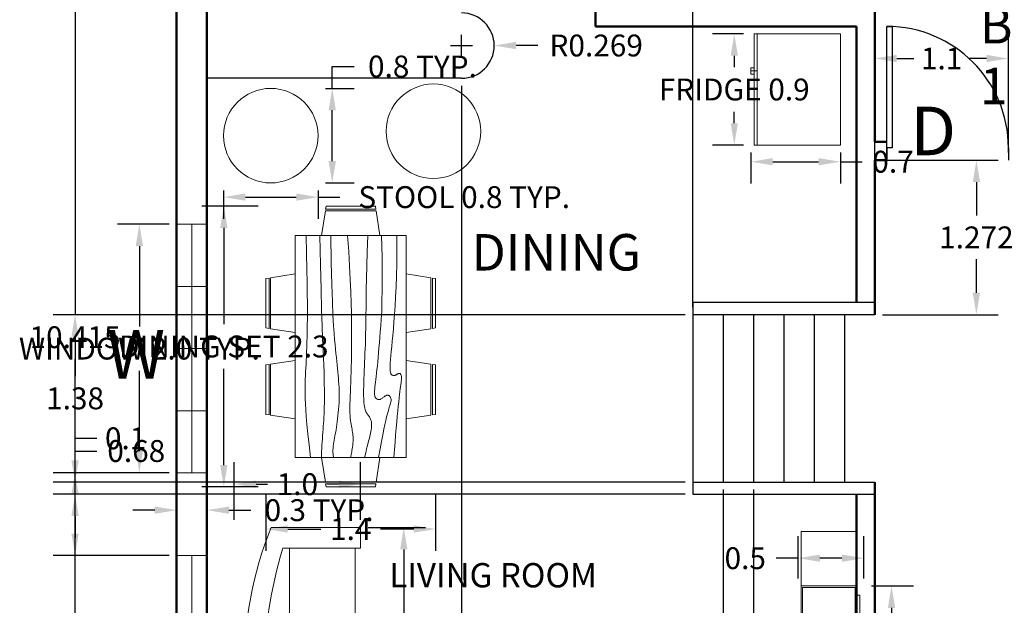
# Model space of a CAD drawing. Units: metres. Extents: x 3.9 to 21.3, y 24.8 to 56.5.
# Tile 4 of 6: x 4.9 to 13, y 31.2 to 36.1. Entities that reach past the tile are written whole.
import ezdxf

# ---------------------------------------------------------------- set-up
doc = ezdxf.new("R2010")
doc.units = ezdxf.units.M
doc.header["$MEASUREMENT"] = 0
for name, color, linetype, lineweight in [('A-AREA-IDEN', 3, 'Continuous', 25), ('A-EQPM', 6, 'Continuous', 18), ('A-FLOR-CASE', 8, 'Continuous', 25), ('A-FLOR-STRS', 7, 'Continuous', 25), ('DIMENSIONS', 2, 'Continuous', 18), ('DOOR', 5, 'Continuous', 25), ('FURNITURE', 6, 'Continuous', 18), ('TEXT', 3, 'Continuous', 18), ('WALL', 1, 'Continuous', 50), ('WINDOW', 4, 'Continuous', 18)]:
    doc.layers.add(name, color=color, linetype=linetype, lineweight=lineweight)
doc.styles.get("Standard").update_dxf_attribs({"font": 'arial.ttf'})
doc.dimstyles.get("Standard").update_dxf_attribs({"dimtxt": 0.18, "dimasz": 0.18, "dimexe": 0.18, "dimexo": 0.0625, "dimgap": 0.09, "dimtad": 0, "dimtih": 1, "dimtoh": 1, "dimdec": 1, "dimzin": 0, "dimdsep": 46, "dimtxsty": 'Standard', "dimcen": 0.09, "dimadec": 0, "dimazin": 0, "dimtfac": 1, "dimtdec": 1, "dimtofl": 0, "dimtmove": 0, "dimatfit": 3, "dimfxl": 1, "dimtolj": 1, "dimtzin": 0, "dimarcsym": 0})

# ---------------------------------------------------------------- blocks, each defined once
blk = doc.blocks.new('*U2')
for p, q in [((0, 0), (0, -100)), ((1000, 0), (1000, -100))]:
    blk.add_line(p, q)
blk.add_lwpolyline([(0, 0), (0, 1000), (43.75, 1000), (43.75, 0)], close=True)
blk.add_arc((0, 0), 1000, 0, 90)
blk = doc.blocks.new('Refrigerator-2 door - 36 in top')
for p, q in [((0, -26.999999), (36, -26.999999)), ((11, -27.999999), (11, -28.999999)), ((12, -26.999999), (12, -28.999999)), ((13, -28.999999), (13, -27.999999)), ((11, -28.999999), (13, -28.999999))]:
    blk.add_line(p, q)
blk.add_lwpolyline([(0, -27.999999), (0, 0), (36, 0), (36, -27.999999)], close=True)
blk = doc.blocks.new('Dining Set - 36 x 72 in.')
for p, q in [((-22.2343, 26.00059), (-23.4847, 17.99762)), ((-22.2304, 26), (-5.7608, 26)), ((-22, 27.5), (-22.1562, 26.50042)), ((-5.8416, 26.5), (-22.1534, 26.5)), ((-22, 27.5), (-6, 27.5)), ((-5.8437, 26.49966), (-6, 27.5)), ((-4.5152, 17.99762), (-5.7655, 25.99926)), ((5.7657, 26.00059), (4.5153, 17.99762)), ((5.7696, 26), (22.2392, 26)), ((6, 27.5), (5.8438, 26.50042)), ((22.1584, 26.5), (5.8466, 26.5)), ((6, 27.5), (22, 27.5)), ((22.1563, 26.49966), (22, 27.5)), ((23.4848, 17.99762), (22.2345, 25.99926)), ((36, 18), (-36, 18)), ((-36, 18), (-36, -18)), ((36, -18), (36, 18)), ((-45.5, 8), (-44.5004, 8.15617)), ((-45.5, 8), (-45.5, -8)), ((-44.5, -8.15843), (-44.5, 8.15338)), ((-44.0006, 8.23428), (-35.9976, 9.48474)), ((-44, 8.23041), (-44, -8.23915)), ((44.0006, 8.23428), (35.9976, 9.48474)), ((44, 8.23041), (44, -8.23915)), ((44.5, -8.15843), (44.5, 8.15338)), ((45.5, 8), (44.5005, 8.15617)), ((45.5, 8), (45.5, -8)), ((-44.4997, -8.15631), (-45.5, -8)), ((-35.9976, -9.48476), (-43.9993, -8.2345)), ((35.9976, -9.48476), (43.9993, -8.2345)), ((44.4997, -8.15631), (45.5, -8)), ((-36, -18), (36, -18)), ((-22.2343, -26.0006), (-23.4847, -17.99762)), ((-4.5152, -17.99762), (-5.7655, -25.99928)), ((5.7657, -26.0006), (4.5153, -17.99762)), ((23.4848, -17.99762), (22.2345, -25.99928)), ((-22.2304, -26), (-5.7608, -26)), ((-22, -27.5), (-22.1562, -26.50044)), ((-5.8416, -26.5), (-22.1534, -26.5)), ((-22, -27.5), (-6, -27.5)), ((-5.8437, -26.49967), (-6, -27.5)), ((5.7696, -26), (22.2392, -26)), ((6, -27.5), (5.8438, -26.50044)), ((22.1584, -26.5), (5.8466, -26.5)), ((6, -27.5), (22, -27.5)), ((22.1563, -26.49967), (22, -27.5))]:
    blk.add_line(p, q)
for points in [[(-36, 15), (-31.1772, 14.97754), (-26.8079, 14.91406), (-22.8538, 14.81543), (-19.276, 14.6875), (-16.0362, 14.53613), (-13.0957, 14.36718), (-10.4159, 14.18652), (-7.9583, 14), (-5.6904, 13.81315), (-3.6035, 13.63021), (-1.6954, 13.45508), (0.0365, 13.29166), (1.5945, 13.14388), (2.9811, 13.01562), (4.1988, 12.9108), (5.25, 12.83333), (6.1393, 12.78613), (6.8802, 12.76823), (7.4883, 12.77767), (7.9792, 12.8125), (8.3685, 12.87077), (8.6719, 12.95052), (8.9049, 13.0498), (9.0833, 13.16666), (9.2205, 13.29899), (9.3216, 13.44401), (9.3895, 13.59879), (9.4271, 13.76041), (9.4373, 13.92594), (9.4232, 14.09245), (9.3875, 14.257), (9.3333, 14.41666), (9.2638, 14.56917), (9.1836, 14.71484), (9.0975, 14.85465), (9.0104, 14.98958), (8.9272, 15.1206), (8.8529, 15.2487), (8.7922, 15.37483), (8.75, 15.5), (8.7305, 15.62467), (8.7344, 15.74739), (8.7617, 15.86621), (8.8125, 15.97916), (8.8867, 16.08431), (8.9844, 16.17968), (9.1055, 16.26334), (9.25, 16.33333), (9.4189, 16.38802), (9.6172, 16.42708), (9.8506, 16.45052), (10.125, 16.45833), (10.4463, 16.45052), (10.8203, 16.42708), (11.2529, 16.38802), (11.75, 16.33333), (12.3184, 16.26318), (12.9694, 16.17838), (13.7151, 16.07991), (14.5677, 15.96875), (15.5395, 15.84586), (16.6426, 15.71224), (17.8893, 15.56884), (19.2917, 15.41666), (20.859, 15.25667), (22.5879, 15.08984), (24.4721, 14.91715), (26.5052, 14.73958), (28.6809, 14.5581), (30.9929, 14.3737), (33.4347, 14.18733), (36, 14)], [(-36, 10), (-28.9766, 10.14274), (-23.1725, 10.20442), (-18.4241, 10.19775), (-14.5677, 10.13541), (-11.4399, 10.03011), (-8.877, 9.89453), (-6.7154, 9.74137), (-4.7917, 9.58333), (-2.9698, 9.43082), (-1.2246, 9.28515), (0.4415, 9.14534), (2.026, 9.01041), (3.5266, 8.87939), (4.9408, 8.7513), (6.266, 8.62516), (7.5, 8.5), (8.6411, 8.37549), (9.6914, 8.2539), (10.6538, 8.13818), (11.5312, 8.03125), (12.3267, 7.93603), (13.043, 7.85547), (13.6831, 7.79248), (14.25, 7.75), (14.7471, 7.7303), (15.1797, 7.73307), (15.5537, 7.75732), (15.875, 7.80208), (16.1494, 7.86637), (16.3828, 7.94922), (16.5811, 8.04964), (16.75, 8.16666), (16.8944, 8.29915), (17.0143, 8.44531), (17.1089, 8.60319), (17.1771, 8.77083), (17.218, 8.94629), (17.2305, 9.1276), (17.2137, 9.31282), (17.1667, 9.5), (17.0895, 9.6875), (16.987, 9.875), (16.8649, 10.0625), (16.7292, 10.25), (16.5856, 10.4375), (16.4401, 10.625), (16.2985, 10.8125), (16.1667, 11), (16.05, 11.18733), (15.9518, 11.3737), (15.8752, 11.5581), (15.8229, 11.73958), (15.798, 11.91715), (15.8034, 12.08984), (15.842, 12.25667), (15.9167, 12.41666), (16.0295, 12.56836), (16.1784, 12.70833), (16.3605, 12.83268), (16.5729, 12.9375), (16.8127, 13.01888), (17.0768, 13.07291), (17.3625, 13.0957), (17.6667, 13.08333), (17.9894, 13.03312), (18.3418, 12.94726), (18.7382, 12.82918), (19.1927, 12.68229), (19.7195, 12.51001), (20.3327, 12.31575), (21.0465, 12.10294), (21.875, 11.875), (22.8357, 11.63354), (23.959, 11.37304), (25.2786, 11.08618), (26.8282, 10.76562), (28.6414, 10.40405), (30.752, 9.99414), (33.1936, 9.52856), (36, 9)], [(-36, 5.5), (-30.7157, 5.3348), (-26.069, 5.20963), (-21.9946, 5.11767), (-18.4271, 5.05208), (-15.3009, 5.00602), (-12.5508, 4.97265), (-10.1112, 4.94515), (-7.9167, 4.91666), (-5.909, 4.88167), (-4.0586, 4.83984), (-2.3429, 4.79215), (-0.7396, 4.73958), (0.7739, 4.6831), (2.22, 4.6237), (3.6213, 4.56233), (5, 4.5), (6.373, 4.43782), (7.7344, 4.3776), (9.0723, 4.32129), (10.375, 4.27083), (11.6309, 4.22819), (12.8281, 4.19531), (13.9551, 4.17415), (15, 4.16666), (15.954, 4.17448), (16.819, 4.19791), (17.6001, 4.23698), (18.3021, 4.29166), (18.9299, 4.36198), (19.4883, 4.44791), (19.9823, 4.54948), (20.4167, 4.66666), (20.7969, 4.79899), (21.1302, 4.94401), (21.4245, 5.09879), (21.6875, 5.26041), (21.9271, 5.42594), (22.1511, 5.59245), (22.3672, 5.757), (22.5834, 5.91666), (22.8065, 6.06868), (23.0404, 6.21093), (23.2879, 6.34147), (23.5521, 6.45833), (23.8358, 6.55957), (24.142, 6.64323), (24.4735, 6.70735), (24.8334, 6.75), (25.2235, 6.76969), (25.642, 6.76692), (26.0858, 6.74267), (26.5521, 6.69791), (27.0379, 6.63362), (27.5404, 6.55078), (28.0565, 6.45036), (28.5834, 6.33333), (29.1242, 6.19987), (29.7071, 6.04687), (30.3661, 5.87044), (31.1354, 5.66666), (32.0493, 5.43164), (33.142, 5.16146), (34.4475, 4.85221), (36, 4.5)], [(-36, -1), (-30.7915, -0.6591), (-26.0195, -0.38216), (-21.6519, -0.16284), (-17.6563, 0.00521), (-14.0005, 0.12833), (-10.6523, 0.21289), (-7.5796, 0.26522), (-4.75, 0.29166), (-2.134, 0.29793), (0.2878, 0.28711), (2.5317, 0.26163), (4.6146, 0.22396), (6.5529, 0.17651), (8.3633, 0.12174), (10.0623, 0.06209), (11.6667, 0), (13.1899, -0.06201), (14.6341, -0.1211), (15.9982, -0.17432), (17.2813, -0.21875), (18.4823, -0.25147), (19.6003, -0.26953), (20.6343, -0.27002), (21.5834, -0.25), (22.4481, -0.20768), (23.2357, -0.14584), (23.9549, -0.06836), (24.6146, 0.02083), (25.2235, 0.11784), (25.7904, 0.21875), (26.3241, 0.31966), (26.8334, 0.41666), (27.3265, 0.50618), (27.8099, 0.58593), (28.2894, 0.65397), (28.7709, 0.70833), (29.2601, 0.74707), (29.763, 0.76823), (30.2855, 0.76985), (30.8334, 0.75), (31.4088, 0.70784), (31.9994, 0.64713), (32.589, 0.57275), (33.1615, 0.48958), (33.7008, 0.4025), (34.1908, 0.3164), (34.6153, 0.23616), (34.9584, 0.16666), (35.2099, 0.11165), (35.3848, 0.07031), (35.504, 0.04069), (35.5886, 0.02083), (35.6594, 0.00879), (35.7377, 0.0026), (35.8442, 0.00032), (36, 0)], [(-36, -6.5), (-27.1843, -6.31267), (-20.084, -6.1263), (-14.469, -5.9419), (-10.1094, -5.76042), (-6.7752, -5.58285), (-4.2363, -5.41016), (-2.2629, -5.24333), (-0.625, -5.08334), (0.8708, -4.93099), (2.2715, -4.78646), (3.5872, -4.64974), (4.8281, -4.52084), (6.0046, -4.39974), (7.127, -4.28646), (8.2053, -4.18099), (9.25, -4.08334), (10.2705, -3.99382), (11.2734, -3.91407), (12.2647, -3.84603), (13.25, -3.79167), (14.2354, -3.75293), (15.2266, -3.73177), (16.2295, -3.73015), (17.25, -3.75), (18.2912, -3.79248), (19.3451, -3.85547), (20.4009, -3.93604), (21.4479, -4.03125), (22.4754, -4.13819), (23.4727, -4.25391), (24.4289, -4.37549), (25.3334, -4.5), (26.1785, -4.62492), (26.9694, -4.74935), (27.7145, -4.87281), (28.4219, -4.99479), (29.1, -5.11483), (29.7572, -5.23242), (30.4016, -5.34709), (31.0417, -5.45834), (31.6837, -5.56437), (32.3262, -5.65821), (32.9658, -5.73153), (33.599, -5.77604), (34.2224, -5.78345), (34.8327, -5.74545), (35.4264, -5.65373), (36, -5.5)], [(-36, -10), (-26.4022, -9.81299), (-18.4675, -9.62891), (-11.9839, -9.45069), (-6.7396, -9.28125), (-2.5226, -9.12354), (0.8789, -8.98047), (3.6769, -8.85498), (6.0833, -8.75), (8.2767, -8.66765), (10.3021, -8.60677), (12.1712, -8.56543), (13.8958, -8.54167), (15.4876, -8.53353), (16.9583, -8.53907), (18.3197, -8.55632), (19.5834, -8.58334), (20.7616, -8.61841), (21.8685, -8.66081), (22.9188, -8.71004), (23.9271, -8.76563), (24.9081, -8.82707), (25.8763, -8.89388), (26.8465, -8.96558), (27.8334, -9.04167), (28.8474, -9.12118), (29.8828, -9.20117), (30.93, -9.27824), (31.9792, -9.34896), (33.0205, -9.40991), (34.0443, -9.45768), (35.0407, -9.48885), (36, -9.5)], [(-36, -14.5), (-30.0881, -14.33513), (-25.0332, -14.21224), (-20.7312, -14.12647), (-17.0781, -14.07292), (-13.97, -14.04671), (-11.3027, -14.04297), (-8.9724, -14.05681), (-6.875, -14.08334), (-4.9224, -14.11833), (-3.0905, -14.16016), (-1.3709, -14.20785), (0.2448, -14.26042), (1.7647, -14.3169), (3.1973, -14.3763), (4.5507, -14.43767), (5.8333, -14.5), (7.0554, -14.5621), (8.235, -14.62175), (9.3922, -14.67652), (10.5469, -14.72396), (11.7192, -14.76164), (12.929, -14.78711), (14.1965, -14.79794), (15.5417, -14.79167), (16.9933, -14.76424), (18.6152, -14.70508), (20.4804, -14.60197), (22.6615, -14.44271), (25.2312, -14.21509), (28.2624, -13.9069), (31.8277, -13.50594), (36, -13)]]:
    blk.add_lwpolyline(points)
blk = doc.blocks.new('Entertainment Center')
for p, q in [((-4, 0), (-5, -1)), ((4, 0), (-4, 0)), ((5, -1), (4, 0)), ((-17, -19), (-17, -1)), ((-17, -1), (43, -1)), ((-16.5, -18.5), (-16.5, -1.5)), ((-16.5, -1.5), (42.5, -1.5)), ((42.5, -1.5), (42.5, -18.5)), ((43, -1), (43, -19)), ((43, -19), (-17, -19)), ((42.5, -18.5), (-16.5, -18.5)), ((-12, -20), (-12, -19)), ((12, -19), (12, -20)), ((15, -20), (15, -19)), ((27, -19), (27, -20)), ((28, -20), (28, -19)), ((40, -19), (40, -20)), ((12, -20), (-12, -20)), ((27, -20), (15, -20)), ((40, -20), (28, -20))]:
    blk.add_line(p, q)
blk.add_arc((0, 40), 61, 259.6111, 280.3889)
blk = doc.blocks.new('Sofa - Roundback 7 ft.')
for p, q in [((-12.00002, -32.4421), (-12.00003, -6.5971)), ((11.99997, -32.4421), (11.99998, -6.5971)), ((-36.000027, -34), (-36.000027, -11.4696)), ((-35.999844, -13.3819), (35.9998, -13.3819)), ((35.99998, -34), (35.99998, -11.4696)), ((-36.000027, -32.4421), (35.99998, -32.4421))]:
    blk.add_line(p, q)
for points in [[(-36.000027, -34), (-42.000027, -34), (-42.000027, -8)], [(41.99998, -8), (41.99998, -34), (35.99998, -34)]]:
    blk.add_lwpolyline(points)
for centre, radius, start, end in [((0, -114.25), 114.25, 68.43141, 111.5686), ((-0.00001, -127.1968), 121.1968, 72.72033, 107.2797)]:
    blk.add_arc(centre, radius, start, end)
blk = doc.blocks.new('WIN-4-LIGHT-2046')
for p, q in [((0.5115, -0.125), (0, -0.125)), ((0.5115, -0.125), (1.0231, -0.125)), ((1.5346, -0.125), (1.0231, -0.125)), ((1.5346, -0.125), (2.0462, -0.125))]:
    blk.add_line(p, q)
for points in [[(0.5115, 0), (0, 0), (0, -0.25), (0.5115, -0.25)], [(0.5115, 0), (1.0231, 0), (1.0231, -0.25), (0.5115, -0.25)], [(1.5346, 0), (1.0231, 0), (1.0231, -0.25), (1.5346, -0.25)], [(1.5346, 0), (2.0462, 0), (2.0462, -0.25), (1.5346, -0.25)]]:
    blk.add_lwpolyline(points, close=True)
blk = doc.blocks.new('STOOL-ROUND-778')
blk.add_circle((0, 0), 0.3891)
blk = doc.blocks.new('*D37')
at = {"layer": 'Defpoints', "color": 0, "transparency": 16777216}
for p in [(6.1571, 34.3672), (5.8502, 32.321), (6.1571, 32.321)]:
    blk.add_point(p, dxfattribs=at)
at = {"layer": 'DIMENSIONS', "color": 0, "lineweight": -2, "transparency": 16777216}
for p, q in [((6.0946, 34.3672), (5.6702, 34.3672)), ((5.8502, 34.1872), (5.8502, 33.5272)), ((5.8502, 32.501), (5.8502, 33.161)), ((6.0946, 32.321), (5.6702, 32.321))]:
    blk.add_line(p, q, dxfattribs=at)
at = {"layer": 'DIMENSIONS', "color": 0, "transparency": 16777216}
for points in [[(5.8202, 34.1872), (5.8802, 34.1872), (5.8502, 34.3672)], [(5.8202, 32.501), (5.8802, 32.501), (5.8502, 32.321)]]:
    blk.add_solid(points, dxfattribs=at)
at = {"layer": 'DIMENSIONS', "color": 0, "transparency": 16777216, "insert": (5.8502, 33.3441), "char_height": 0.18, "attachment_point": 5}
blk.add_mtext('\\A1;WINDOW 2.0 TYP.', dxfattribs=at)
blk = doc.blocks.new('*D38')
at = {"layer": 'Defpoints', "color": 0, "transparency": 16777216}
for p in [(6.1571, 32.321), (6.4071, 32.321), (6.4071, 32.0141)]:
    blk.add_point(p, dxfattribs=at)
at = {"layer": 'DIMENSIONS', "color": 0, "lineweight": -2, "transparency": 16777216}
for p, q in [((6.1571, 32.2585), (6.1571, 31.8341)), ((6.4071, 32.2585), (6.4071, 31.8341)), ((5.9771, 32.0141), (5.7971, 32.0141)), ((6.5871, 32.0141), (6.7671, 32.0141))]:
    blk.add_line(p, q, dxfattribs=at)
at = {"layer": 'DIMENSIONS', "color": 0, "transparency": 16777216}
for points in [[(5.9771, 32.0441), (5.9771, 31.9841), (6.1571, 32.0141)], [(6.5871, 32.0441), (6.5871, 31.9841), (6.4071, 32.0141)]]:
    blk.add_solid(points, dxfattribs=at)
at = {"layer": 'DIMENSIONS', "color": 0, "transparency": 16777216, "insert": (7.3301, 32.0141), "char_height": 0.18, "attachment_point": 5}
blk.add_mtext('\\A1;0.3 TYP.', dxfattribs=at)
blk = doc.blocks.new('*D49')
at = {"layer": 'Defpoints', "color": 0, "transparency": 16777216}
for p in [(6.5435, 34.7074), (7.3217, 34.7074), (7.3217, 34.5907)]:
    blk.add_point(p, dxfattribs=at)
at = {"layer": 'DIMENSIONS', "color": 0, "lineweight": -2, "transparency": 16777216}
for p, q in [((6.5435, 34.6449), (6.5435, 34.4107)), ((7.3217, 34.6449), (7.3217, 34.4107)), ((6.7235, 34.5907), (7.1417, 34.5907)), ((7.3217, 34.5907), (7.5017, 34.5907))]:
    blk.add_line(p, q, dxfattribs=at)
at = {"layer": 'DIMENSIONS', "color": 0, "transparency": 16777216}
for points in [[(6.7235, 34.6207), (6.7235, 34.5607), (6.5435, 34.5907)], [(7.1417, 34.6207), (7.1417, 34.5607), (7.3217, 34.5907)]]:
    blk.add_solid(points, dxfattribs=at)
at = {"layer": 'DIMENSIONS', "color": 0, "transparency": 16777216, "insert": (8.5254, 34.5907), "char_height": 0.18, "attachment_point": 5}
blk.add_mtext('\\A1;STOOL 0.8 TYP.', dxfattribs=at)
blk = doc.blocks.new('*D50')
at = {"layer": 'Defpoints', "color": 0, "transparency": 16777216}
for p in [(7.3217, 35.4856), (7.4385, 35.4856), (7.3217, 34.7074)]:
    blk.add_point(p, dxfattribs=at)
at = {"layer": 'DIMENSIONS', "color": 0, "lineweight": -2, "transparency": 16777216}
for p, q in [((7.4385, 35.4856), (7.4385, 35.6656)), ((7.4385, 35.6656), (7.6185, 35.6656)), ((7.3842, 35.4856), (7.6185, 35.4856)), ((7.4385, 34.8874), (7.4385, 35.3056)), ((7.3842, 34.7074), (7.6185, 34.7074))]:
    blk.add_line(p, q, dxfattribs=at)
at = {"layer": 'DIMENSIONS', "color": 0, "transparency": 16777216}
for points in [[(7.4085, 35.3056), (7.4685, 35.3056), (7.4385, 35.4856)], [(7.4085, 34.8874), (7.4685, 34.8874), (7.4385, 34.7074)]]:
    blk.add_solid(points, dxfattribs=at)
at = {"layer": 'DIMENSIONS', "color": 0, "transparency": 16777216, "insert": (8.1815, 35.6656), "char_height": 0.18, "attachment_point": 5}
blk.add_mtext('\\A1;0.8 TYP.', dxfattribs=at)
blk = doc.blocks.new('*D51')
at = {"layer": 'Defpoints', "color": 0, "transparency": 16777216}
for p in [(10.8867, 35.9335), (10.7495, 35.0191), (10.8867, 35.0191)]:
    blk.add_point(p, dxfattribs=at)
at = {"layer": 'DIMENSIONS', "color": 0, "lineweight": -2, "transparency": 16777216}
for p, q in [((10.8242, 35.9335), (10.5695, 35.9335)), ((10.7495, 35.7535), (10.7495, 35.6594)), ((10.7495, 35.1991), (10.7495, 35.2933)), ((10.8242, 35.0191), (10.5695, 35.0191))]:
    blk.add_line(p, q, dxfattribs=at)
at = {"layer": 'DIMENSIONS', "color": 0, "transparency": 16777216}
for points in [[(10.7195, 35.7535), (10.7795, 35.7535), (10.7495, 35.9335)], [(10.7195, 35.1991), (10.7795, 35.1991), (10.7495, 35.0191)]]:
    blk.add_solid(points, dxfattribs=at)
at = {"layer": 'DIMENSIONS', "color": 0, "transparency": 16777216, "insert": (10.7495, 35.4763), "char_height": 0.18, "attachment_point": 5}
blk.add_mtext('\\A1;FRIDGE 0.9', dxfattribs=at)
blk = doc.blocks.new('*D52')
at = {"layer": 'Defpoints', "color": 0, "transparency": 16777216}
for p in [(10.8867, 35.0191), (11.6233, 35.0191), (11.6233, 34.882)]:
    blk.add_point(p, dxfattribs=at)
at = {"layer": 'DIMENSIONS', "color": 0, "lineweight": -2, "transparency": 16777216}
for p, q in [((10.8867, 34.9566), (10.8867, 34.702)), ((11.6233, 34.9566), (11.6233, 34.702)), ((11.0667, 34.882), (11.4433, 34.882)), ((11.6233, 34.882), (11.8033, 34.882))]:
    blk.add_line(p, q, dxfattribs=at)
at = {"layer": 'DIMENSIONS', "color": 0, "transparency": 16777216}
for points in [[(11.0667, 34.912), (11.0667, 34.852), (10.8867, 34.882)], [(11.4433, 34.912), (11.4433, 34.852), (11.6233, 34.882)]]:
    blk.add_solid(points, dxfattribs=at)
at = {"layer": 'DIMENSIONS', "color": 0, "transparency": 16777216, "insert": (12.0571, 34.882), "char_height": 0.18, "attachment_point": 5}
blk.add_mtext('\\A1;0.7', dxfattribs=at)
blk = doc.blocks.new('*D57')
at = {"layer": 'Defpoints', "color": 0, "transparency": 16777216}
for p in [(6.8924, 34.5172), (6.5457, 32.2058), (6.8924, 32.2058)]:
    blk.add_point(p, dxfattribs=at)
at = {"layer": 'DIMENSIONS', "color": 0, "lineweight": -2, "transparency": 16777216}
for p, q in [((6.8299, 34.5172), (6.3657, 34.5172)), ((6.5457, 34.3372), (6.5457, 33.5447)), ((6.5457, 32.3858), (6.5457, 33.1784)), ((6.8299, 32.2058), (6.3657, 32.2058))]:
    blk.add_line(p, q, dxfattribs=at)
at = {"layer": 'DIMENSIONS', "color": 0, "transparency": 16777216}
for points in [[(6.5157, 34.3372), (6.5757, 34.3372), (6.5457, 34.5172)], [(6.5157, 32.3858), (6.5757, 32.3858), (6.5457, 32.2058)]]:
    blk.add_solid(points, dxfattribs=at)
at = {"layer": 'DIMENSIONS', "color": 0, "transparency": 16777216, "insert": (6.5457, 33.3615), "char_height": 0.18, "attachment_point": 5}
blk.add_mtext('\\A1;DINING SET 2.3', dxfattribs=at)
blk = doc.blocks.new('*D58')
at = {"layer": 'Defpoints', "color": 0, "transparency": 16777216}
for p in [(6.8924, 32.2058), (8.2894, 32.2058), (8.2894, 31.8591)]:
    blk.add_point(p, dxfattribs=at)
at = {"layer": 'DIMENSIONS', "color": 0, "lineweight": -2, "transparency": 16777216}
for p, q in [((6.8924, 32.1433), (6.8924, 31.6791)), ((8.2894, 32.1433), (8.2894, 31.6791)), ((7.0724, 31.8591), (7.3459, 31.8591)), ((8.1094, 31.8591), (7.8359, 31.8591))]:
    blk.add_line(p, q, dxfattribs=at)
at = {"layer": 'DIMENSIONS', "color": 0, "transparency": 16777216}
for points in [[(7.0724, 31.8891), (7.0724, 31.8291), (6.8924, 31.8591)], [(8.1094, 31.8891), (8.1094, 31.8291), (8.2894, 31.8591)]]:
    blk.add_solid(points, dxfattribs=at)
at = {"layer": 'DIMENSIONS', "color": 0, "transparency": 16777216, "insert": (7.5909, 31.8591), "char_height": 0.18, "attachment_point": 5}
blk.add_mtext('\\A1;1.4', dxfattribs=at)
blk = doc.blocks.new('*D59')
at = {"layer": 'Defpoints', "color": 0, "transparency": 16777216}
for p in [(11.8164, 31.3903), (12.045, 31.3903), (11.8164, 29.8663)]:
    blk.add_point(p, dxfattribs=at)
at = {"layer": 'DIMENSIONS', "color": 0, "lineweight": -2, "transparency": 16777216}
for p, q in [((11.8789, 31.3903), (12.225, 31.3903)), ((12.045, 31.2103), (12.045, 30.8102)), ((12.045, 30.0463), (12.045, 30.4464)), ((11.8789, 29.8663), (12.225, 29.8663))]:
    blk.add_line(p, q, dxfattribs=at)
at = {"layer": 'DIMENSIONS', "color": 0, "transparency": 16777216}
for points in [[(12.015, 31.2103), (12.075, 31.2103), (12.045, 31.3903)], [(12.015, 30.0463), (12.075, 30.0463), (12.045, 29.8663)]]:
    blk.add_solid(points, dxfattribs=at)
at = {"layer": 'DIMENSIONS', "color": 0, "transparency": 16777216, "insert": (12.045, 30.6283), "char_height": 0.18, "attachment_point": 5}
blk.add_mtext('\\A1;MEDIA UNIT 1.5', dxfattribs=at)
blk = doc.blocks.new('*D60')
at = {"layer": 'Defpoints', "color": 0, "transparency": 16777216}
for p in [(11.2746, 31.6189), (11.2746, 31.3903), (11.8164, 31.3903)]:
    blk.add_point(p, dxfattribs=at)
at = {"layer": 'DIMENSIONS', "color": 0, "lineweight": -2, "transparency": 16777216}
for p, q in [((11.2746, 31.4528), (11.2746, 31.7989)), ((11.8164, 31.4528), (11.8164, 31.7989)), ((11.2746, 31.6189), (11.0946, 31.6189)), ((11.6364, 31.6189), (11.4546, 31.6189))]:
    blk.add_line(p, q, dxfattribs=at)
at = {"layer": 'DIMENSIONS', "color": 0, "transparency": 16777216}
for points in [[(11.4546, 31.6489), (11.4546, 31.5889), (11.2746, 31.6189)], [(11.6364, 31.6489), (11.6364, 31.5889), (11.8164, 31.6189)]]:
    blk.add_solid(points, dxfattribs=at)
at = {"layer": 'DIMENSIONS', "color": 0, "transparency": 16777216, "insert": (10.84, 31.6189), "char_height": 0.18, "attachment_point": 5}
blk.add_mtext('\\A1;0.5', dxfattribs=at)
blk = doc.blocks.new('*D61')
at = {"layer": 'Defpoints', "color": 0, "transparency": 16777216}
for p in [(7.6708, 31.8712), (8.0277, 31.8712), (7.6708, 29.4918)]:
    blk.add_point(p, dxfattribs=at)
at = {"layer": 'DIMENSIONS', "color": 0, "lineweight": -2, "transparency": 16777216}
for p, q in [((7.7333, 31.8712), (8.2077, 31.8712)), ((8.0277, 31.6912), (8.0277, 30.8646)), ((8.0277, 29.6718), (8.0277, 30.4984)), ((7.7333, 29.4918), (8.2077, 29.4918))]:
    blk.add_line(p, q, dxfattribs=at)
at = {"layer": 'DIMENSIONS', "color": 0, "transparency": 16777216}
for points in [[(7.9977, 31.6912), (8.0577, 31.6912), (8.0277, 31.8712)], [(7.9977, 29.6718), (8.0577, 29.6718), (8.0277, 29.4918)]]:
    blk.add_solid(points, dxfattribs=at)
at = {"layer": 'DIMENSIONS', "color": 0, "transparency": 16777216, "insert": (8.0277, 30.6815), "char_height": 0.18, "attachment_point": 5}
blk.add_mtext('\\A1;SOFA 2.4', dxfattribs=at)
blk = doc.blocks.new('*D62')
at = {"layer": 'Defpoints', "color": 0, "transparency": 16777216}
for p in [(6.6321, 32.2281), (6.6321, 31.8712), (7.6708, 31.8712)]:
    blk.add_point(p, dxfattribs=at)
at = {"layer": 'DIMENSIONS', "color": 0, "lineweight": -2, "transparency": 16777216}
for p, q in [((6.6321, 31.9337), (6.6321, 32.4081)), ((7.6708, 31.9337), (7.6708, 32.4081)), ((6.8121, 32.2281), (6.9064, 32.2281)), ((7.4908, 32.2281), (7.3965, 32.2281))]:
    blk.add_line(p, q, dxfattribs=at)
at = {"layer": 'DIMENSIONS', "color": 0, "transparency": 16777216}
for points in [[(6.8121, 32.2581), (6.8121, 32.1981), (6.6321, 32.2281)], [(7.4908, 32.2581), (7.4908, 32.1981), (7.6708, 32.2281)]]:
    blk.add_solid(points, dxfattribs=at)
at = {"layer": 'DIMENSIONS', "color": 0, "transparency": 16777216, "insert": (7.1514, 32.2281), "char_height": 0.18, "attachment_point": 5}
blk.add_mtext('\\A1;1.0', dxfattribs=at)
blk = doc.blocks.new('*D65')
at = {"layer": 'Defpoints', "color": 0, "transparency": 16777216}
for p in [(9.0686, 30.8635), (9.1864, 30.8635), (9.0686, 30.0783)]:
    blk.add_point(p, dxfattribs=at)
at = {"layer": 'DIMENSIONS', "color": 0, "lineweight": -2, "transparency": 16777216}
for p, q in [((9.1864, 30.8635), (9.1864, 31.0435)), ((9.1864, 31.0435), (9.3664, 31.0435)), ((9.1311, 30.8635), (9.3664, 30.8635)), ((9.1864, 30.2583), (9.1864, 30.6835)), ((9.1311, 30.0783), (9.3664, 30.0783))]:
    blk.add_line(p, q, dxfattribs=at)
at = {"layer": 'DIMENSIONS', "color": 0, "transparency": 16777216}
for points in [[(9.1564, 30.6835), (9.2164, 30.6835), (9.1864, 30.8635)], [(9.1564, 30.2583), (9.2164, 30.2583), (9.1864, 30.0783)]]:
    blk.add_solid(points, dxfattribs=at)
at = {"layer": 'DIMENSIONS', "color": 0, "transparency": 16777216, "insert": (10.5975, 31.0435), "char_height": 0.18, "attachment_point": 5}
blk.add_mtext('\\A1;COFFEE TABLE 0.8', dxfattribs=at)
blk = doc.blocks.new('*D75')
at = {"layer": 'Defpoints', "color": 0, "transparency": 16777216}
for p in [(13.0071, 35.7316), (11.9071, 34.8951), (13.0071, 34.8951)]:
    blk.add_point(p, dxfattribs=at)
at = {"layer": 'DIMENSIONS', "color": 0, "lineweight": -2, "transparency": 16777216}
for p, q in [((11.9071, 34.9576), (11.9071, 35.9116)), ((13.0071, 34.9576), (13.0071, 35.9116)), ((12.0871, 35.7316), (12.2291, 35.7316)), ((12.8271, 35.7316), (12.6851, 35.7316))]:
    blk.add_line(p, q, dxfattribs=at)
at = {"layer": 'DIMENSIONS', "color": 0, "transparency": 16777216}
for points in [[(12.0871, 35.7616), (12.0871, 35.7016), (11.9071, 35.7316)], [(12.8271, 35.7616), (12.8271, 35.7016), (13.0071, 35.7316)]]:
    blk.add_solid(points, dxfattribs=at)
at = {"layer": 'DIMENSIONS', "color": 0, "transparency": 16777216, "insert": (12.4571, 35.7316), "char_height": 0.18, "attachment_point": 5}
blk.add_mtext('\\A1;1.1', dxfattribs=at)
blk = doc.blocks.new('*D76')
at = {"layer": 'Defpoints', "color": 0, "transparency": 16777216}
for p in [(6.4071, 38.6451), (5.3206, 28.2303), (6.4071, 28.2303)]:
    blk.add_point(p, dxfattribs=at)
at = {"layer": 'DIMENSIONS', "color": 0, "lineweight": -2, "transparency": 16777216}
for p, q in [((6.3446, 38.6451), (5.1406, 38.6451)), ((5.3206, 38.4651), (5.3206, 33.6196)), ((5.3206, 28.4103), (5.3206, 33.2558)), ((6.3446, 28.2303), (5.1406, 28.2303))]:
    blk.add_line(p, q, dxfattribs=at)
at = {"layer": 'DIMENSIONS', "color": 0, "transparency": 16777216}
for points in [[(5.2906, 38.4651), (5.3506, 38.4651), (5.3206, 38.6451)], [(5.2906, 28.4103), (5.3506, 28.4103), (5.3206, 28.2303)]]:
    blk.add_solid(points, dxfattribs=at)
at = {"layer": 'DIMENSIONS', "color": 0, "transparency": 16777216, "insert": (5.3206, 33.4377), "char_height": 0.18, "attachment_point": 5}
blk.add_mtext('\\A1;10.415', dxfattribs=at)
blk = doc.blocks.new('*D77')
at = {"layer": 'Defpoints', "color": 0, "transparency": 16777216}
for p in [(11.9071, 40.5816), (10.4071, 33.623), (11.9071, 33.623)]:
    blk.add_point(p, dxfattribs=at)
at = {"layer": 'DIMENSIONS', "color": 0, "lineweight": -2, "transparency": 16777216}
for p, q in [((10.4071, 33.6855), (10.4071, 40.7616)), ((11.9071, 33.6855), (11.9071, 40.7616)), ((10.5871, 40.5816), (10.9111, 40.5816)), ((11.7271, 40.5816), (11.4032, 40.5816))]:
    blk.add_line(p, q, dxfattribs=at)
at = {"layer": 'DIMENSIONS', "color": 0, "transparency": 16777216}
for points in [[(10.5871, 40.6116), (10.5871, 40.5516), (10.4071, 40.5816)], [(11.7271, 40.6116), (11.7271, 40.5516), (11.9071, 40.5816)]]:
    blk.add_solid(points, dxfattribs=at)
at = {"layer": 'DIMENSIONS', "color": 0, "transparency": 16777216, "insert": (11.1571, 40.5816), "char_height": 0.18, "attachment_point": 5}
blk.add_mtext('\\A1;1.5', dxfattribs=at)
blk = doc.blocks.new('*D78')
at = {"layer": 'Defpoints', "color": 0, "transparency": 16777216}
for p in [(10.4071, 33.623), (5.3206, 32.2457), (10.4071, 32.2457)]:
    blk.add_point(p, dxfattribs=at)
at = {"layer": 'DIMENSIONS', "color": 0, "lineweight": -2, "transparency": 16777216}
for p, q in [((10.3446, 33.623), (5.1406, 33.623)), ((5.3206, 33.443), (5.3206, 33.1163)), ((5.3206, 32.4257), (5.3206, 32.7524)), ((10.3446, 32.2457), (5.1406, 32.2457))]:
    blk.add_line(p, q, dxfattribs=at)
at = {"layer": 'DIMENSIONS', "color": 0, "transparency": 16777216}
for points in [[(5.2906, 33.443), (5.3506, 33.443), (5.3206, 33.623)], [(5.2906, 32.4257), (5.3506, 32.4257), (5.3206, 32.2457)]]:
    blk.add_solid(points, dxfattribs=at)
at = {"layer": 'DIMENSIONS', "color": 0, "transparency": 16777216, "insert": (5.3206, 32.9343), "char_height": 0.18, "attachment_point": 5}
blk.add_mtext('\\A1;1.38', dxfattribs=at)
blk = doc.blocks.new('*D79')
at = {"layer": 'Defpoints', "color": 0, "transparency": 16777216}
for p in [(10.6571, 32.2457), (10.9071, 32.2457), (10.9071, 25.0086)]:
    blk.add_point(p, dxfattribs=at)
at = {"layer": 'DIMENSIONS', "color": 0, "lineweight": -2, "transparency": 16777216}
for p, q in [((10.6571, 32.1832), (10.6571, 24.8286)), ((10.9071, 32.1832), (10.9071, 24.8286)), ((10.4771, 25.0086), (10.2971, 25.0086)), ((11.0871, 25.0086), (11.2671, 25.0086))]:
    blk.add_line(p, q, dxfattribs=at)
at = {"layer": 'DIMENSIONS', "color": 0, "transparency": 16777216}
for points in [[(10.4771, 25.0386), (10.4771, 24.9786), (10.6571, 25.0086)], [(11.0871, 25.0386), (11.0871, 24.9786), (10.9071, 25.0086)]]:
    blk.add_solid(points, dxfattribs=at)
at = {"layer": 'DIMENSIONS', "color": 0, "transparency": 16777216, "insert": (11.5916, 25.0086), "char_height": 0.18, "attachment_point": 5}
blk.add_mtext('\\A1;0.25', dxfattribs=at)
blk = doc.blocks.new('*D80')
at = {"layer": 'Defpoints', "color": 0, "transparency": 16777216}
for p in [(5.3206, 32.2457), (10.4071, 32.2457), (10.4071, 32.1457)]:
    blk.add_point(p, dxfattribs=at)
at = {"layer": 'DIMENSIONS', "color": 0, "lineweight": -2, "transparency": 16777216}
for p, q in [((5.3206, 32.4257), (5.3206, 32.6057)), ((5.3206, 32.6057), (5.5006, 32.6057)), ((10.3446, 32.2457), (5.1406, 32.2457)), ((10.3446, 32.1457), (5.1406, 32.1457)), ((5.3206, 31.9657), (5.3206, 31.7857))]:
    blk.add_line(p, q, dxfattribs=at)
at = {"layer": 'DIMENSIONS', "color": 0, "transparency": 16777216}
for points in [[(5.2906, 32.4257), (5.3506, 32.4257), (5.3206, 32.2457)], [(5.2906, 31.9657), (5.3506, 31.9657), (5.3206, 32.1457)]]:
    blk.add_solid(points, dxfattribs=at)
at = {"layer": 'DIMENSIONS', "color": 0, "transparency": 16777216, "insert": (5.7371, 32.6057), "char_height": 0.18, "attachment_point": 5}
blk.add_mtext('\\A1;0.1', dxfattribs=at)
blk = doc.blocks.new('*D92')
at = {"layer": 'Defpoints', "color": 0, "transparency": 16777216}
for p in [(5.3206, 32.321), (6.1571, 32.321), (6.1571, 31.6409)]:
    blk.add_point(p, dxfattribs=at)
at = {"layer": 'DIMENSIONS', "color": 0, "lineweight": -2, "transparency": 16777216}
for p, q in [((5.3206, 32.321), (5.3206, 32.501)), ((5.3206, 32.501), (5.5006, 32.501)), ((6.0946, 32.321), (5.1406, 32.321)), ((5.3206, 31.8209), (5.3206, 32.141)), ((6.0946, 31.6409), (5.1406, 31.6409))]:
    blk.add_line(p, q, dxfattribs=at)
at = {"layer": 'DIMENSIONS', "color": 0, "transparency": 16777216}
for points in [[(5.2906, 32.141), (5.3506, 32.141), (5.3206, 32.321)], [(5.2906, 31.8209), (5.3506, 31.8209), (5.3206, 31.6409)]]:
    blk.add_solid(points, dxfattribs=at)
at = {"layer": 'DIMENSIONS', "color": 0, "transparency": 16777216, "insert": (5.8246, 32.501), "char_height": 0.18, "attachment_point": 5}
blk.add_mtext('\\A1;0.68', dxfattribs=at)
blk = doc.blocks.new('*D96')
at = {"layer": 'Defpoints', "color": 0, "transparency": 16777216}
for p in [(6.4071, 35.5686), (8.5033, 35.5686), (8.5033, 25.0086)]:
    blk.add_point(p, dxfattribs=at)
at = {"layer": 'DIMENSIONS', "color": 0, "lineweight": -2, "transparency": 16777216}
for p, q in [((6.4071, 35.5061), (6.4071, 24.8286)), ((8.5033, 35.5061), (8.5033, 24.8286)), ((6.5871, 25.0086), (7.06, 25.0086)), ((8.3233, 25.0086), (7.8504, 25.0086))]:
    blk.add_line(p, q, dxfattribs=at)
at = {"layer": 'DIMENSIONS', "color": 0, "transparency": 16777216}
for points in [[(6.5871, 25.0386), (6.5871, 24.9786), (6.4071, 25.0086)], [(8.3233, 25.0386), (8.3233, 24.9786), (8.5033, 25.0086)]]:
    blk.add_solid(points, dxfattribs=at)
at = {"layer": 'DIMENSIONS', "color": 0, "transparency": 16777216, "insert": (7.4552, 25.0086), "char_height": 0.18, "attachment_point": 5}
blk.add_mtext('\\A1;2.096', dxfattribs=at)
blk = doc.blocks.new('*D102')
at = {"layer": 'Defpoints', "color": 0, "transparency": 16777216}
for p in [(11.9071, 34.8951), (11.9071, 33.623), (12.7436, 33.623)]:
    blk.add_point(p, dxfattribs=at)
at = {"layer": 'DIMENSIONS', "color": 0, "lineweight": -2, "transparency": 16777216}
for p, q in [((11.9696, 34.8951), (12.9236, 34.8951)), ((12.7436, 34.7151), (12.7436, 34.4394)), ((12.7436, 33.803), (12.7436, 34.0787)), ((11.9696, 33.623), (12.9236, 33.623))]:
    blk.add_line(p, q, dxfattribs=at)
at = {"layer": 'DIMENSIONS', "color": 0, "transparency": 16777216}
for points in [[(12.7136, 34.7151), (12.7736, 34.7151), (12.7436, 34.8951)], [(12.7136, 33.803), (12.7736, 33.803), (12.7436, 33.623)]]:
    blk.add_solid(points, dxfattribs=at)
at = {"layer": 'DIMENSIONS', "color": 0, "transparency": 16777216, "insert": (12.7436, 34.2591), "char_height": 0.18, "attachment_point": 5}
blk.add_mtext('\\A1;1.272', dxfattribs=at)
blk = doc.blocks.new('*D106')
at = {"layer": 'Defpoints', "color": 0, "transparency": 16777216}
for p in [(8.5033, 35.8376), (8.7723, 35.838)]:
    blk.add_point(p, dxfattribs=at)
at = {"layer": 'DIMENSIONS', "color": 0, "lineweight": -2, "transparency": 16777216}
for p, q in [((8.5033, 35.7476), (8.5033, 35.9276)), ((8.4133, 35.8376), (8.5933, 35.8376)), ((9.1323, 35.8385), (8.9523, 35.8383))]:
    blk.add_line(p, q, dxfattribs=at)
at = {"layer": 'DIMENSIONS', "color": 0, "transparency": 16777216}
blk.add_solid([(8.9522, 35.8683), (8.9523, 35.8083), (8.7723, 35.838)], dxfattribs=at)
at = {"layer": 'DIMENSIONS', "color": 0, "transparency": 16777216, "insert": (9.6123, 35.8385), "char_height": 0.18, "attachment_point": 5}
blk.add_mtext('\\A1;R0.269', dxfattribs=at)

msp = doc.modelspace()

# ---------------------------------------------------------------- linework, layer by layer
at = {"layer": 'A-FLOR-CASE'}
msp.add_line((8.5033, 35.5686), (6.4071, 35.5686), dxfattribs=at)
msp.add_arc((8.5033, 35.8376), 0.269, 270, 90, dxfattribs=at)
at = {"layer": 'A-FLOR-STRS'}
for p, q in [((11.9071, 33.723), (10.4071, 33.723)), ((10.4071, 33.723), (10.4071, 32.1457)), ((11.9071, 33.623), (10.4071, 33.623)), ((10.6571, 33.623), (10.6571, 32.2457)), ((10.9071, 33.623), (10.9071, 32.2457)), ((11.1571, 33.623), (11.1571, 32.2457)), ((11.4071, 33.623), (11.4071, 32.2457)), ((11.6571, 33.623), (11.6571, 32.2457)), ((10.4071, 32.2457), (11.9071, 32.2457)), ((10.4071, 32.1457), (11.9071, 32.1457))]:
    msp.add_line(p, q, dxfattribs=at)
at = {"layer": 'DOOR'}
msp.add_line((12.0071, 34.8951), (12.0071, 35.0451), dxfattribs=at)
at = {"layer": 'FURNITURE'}
msp.add_lwpolyline([(11.3, 31.3903), (11.7571, 31.3903), (11.7571, 31.8386), (11.3, 31.8386)], close=True, dxfattribs=at)
at = {"layer": 'WALL'}
for p, q in [((6.1571, 25.8451), (6.1571, 38.8951)), ((6.4071, 28.2303), (6.4071, 38.6451)), ((9.6071, 35.9951), (9.6071, 38.6451)), ((11.9071, 35.0451), (11.9071, 37.2672)), ((9.6071, 35.9951), (11.7571, 35.9951)), ((11.7571, 33.723), (11.7571, 35.9951)), ((11.9071, 35.0451), (12.0071, 35.0451)), ((11.9071, 34.8951), (12.0071, 34.8951)), ((11.9071, 33.623), (11.9071, 34.8951)), ((11.9071, 29.1451), (11.9071, 32.2457)), ((11.7571, 28.2303), (11.7571, 32.1457))]:
    msp.add_line(p, q, dxfattribs=at)

# ---------------------------------------------------------------- block references
at = {"layer": 'A-EQPM', "xscale": 0.0254, "yscale": 0.0254, "zscale": 0.0254, "rotation": 270}
msp.add_blockref('Refrigerator-2 door - 36 in top', (11.6233, 35.9335), dxfattribs=at)
at = {"layer": 'DOOR', "xscale": 0.001, "yscale": 0.001, "zscale": 0.001}
msp.add_blockref('*U2', (12.0071, 34.9951), dxfattribs=at)
at = {"layer": 'FURNITURE'}
for p in [(8.2721, 35.1327), (6.9326, 35.0965)]:
    msp.add_blockref('STOOL-ROUND-778', p, dxfattribs=at)
for name, p, xscale, yscale, zscale, rotation in [('Dining Set - 36 x 72 in.', (7.5909, 33.3615), 0.0254, 0.0254, 0.0254, 270), ('Sofa - Roundback 7 ft.', (6.7077, 30.6815), 0.0283257265101147, 0.0283257265101147, 0.0283257265101147, 89.99997936313675), ('Entertainment Center', (11.2746, 30.2981), 0.0254, 0.0254, 0.0254, 90)]:
    msp.add_blockref(name, p, dxfattribs=dict(at, xscale=xscale, yscale=yscale, zscale=zscale, rotation=rotation))
at = {"layer": 'WINDOW', "rotation": 269.9999999999997}
for p in [(6.4071, 34.3672), (6.4071, 31.6409)]:
    msp.add_blockref('WIN-4-LIGHT-2046', p, dxfattribs=at)

# ---------------------------------------------------------------- texts
at = {"layer": 'A-AREA-IDEN', "attachment_point": 1}
for s, width, insert, char_height in [('BEDROOM 1', 1.45972, (12.7722, 36.1551), 0.3), ('DINING ', 1.252017, (8.5857, 34.2866), 0.3), ('LIVING ROOM', 2.121341, (7.9075, 31.5788), 0.2)]:
    msp.add_mtext_dynamic_manual_height_columns(s, width=width, gutter_width=1, heights=[0], dxfattribs=dict(at, insert=insert, char_height=char_height))
at = {"layer": 'TEXT', "char_height": 0.4, "attachment_point": 1}
for s, insert in [('D', (12.2005, 35.3355)), ('W', (5.583, 33.4969))]:
    msp.add_mtext_dynamic_manual_height_columns(s, width=0.69425, gutter_width=1, heights=[0], dxfattribs=dict(at, insert=insert))

# ---------------------------------------------------------------- dimensions: what is measured, and where the dimension line sits
at = {"layer": 'DIMENSIONS'}
for base, p1, p2, override, picture, middle in [((11.9071, 40.5816), (10.4071, 33.623), (11.9071, 33.623), {"dimdec": 1, "dimlfac": 1, "dimrnd": 0, "dimzin": 0, "dimdsep": 46, "dimlunit": 2}, '*D77', (11.1571, 40.5816)), ((13.0071, 35.7316), (11.9071, 34.8951), (13.0071, 34.8951), {"dimdec": 1, "dimlfac": 1, "dimrnd": 0, "dimzin": 0, "dimdsep": 46, "dimlunit": 2}, '*D75', (12.4571, 35.7316)), ((8.5033, 25.0086), (6.4071, 35.5686), (8.5033, 35.5686), {"dimdec": 3, "dimlfac": 1, "dimrnd": 0, "dimzin": 0, "dimdsep": 46, "dimlunit": 2}, '*D96', (7.4552, 25.0086)), ((11.6233, 34.882), (10.8867, 35.0191), (11.6233, 35.0191), {"dimdec": 1, "dimlfac": 1, "dimrnd": 0, "dimzin": 0, "dimdsep": 46, "dimlunit": 2}, '*D52', (12.0571, 34.882)), ((8.2894, 31.8591), (6.8924, 32.2058), (8.2894, 32.2058), {"dimdec": 1, "dimlfac": 1, "dimrnd": 0, "dimzin": 0, "dimdsep": 46, "dimlunit": 2}, '*D58', (7.5909, 31.8591)), ((10.9071, 25.0086), (10.6571, 32.2457), (10.9071, 32.2457), {"dimdec": 2, "dimlfac": 1, "dimrnd": 0, "dimzin": 0, "dimdsep": 46, "dimlunit": 2}, '*D79', (11.5916, 25.0086))]:
    dim = msp.add_linear_dim(base=base, p1=p1, p2=p2, dimstyle='Standard', override=override, dxfattribs=at)
    dim.commit()
    dim.dimension.update_dxf_attribs({"geometry": picture, "text_midpoint": middle})
for base, p1, p2, angle, override, picture, middle in [((5.3206, 28.2303), (6.4071, 38.6451), (6.4071, 28.2303), 90, {"dimdec": 3, "dimlfac": 1, "dimrnd": 0, "dimzin": 0, "dimdsep": 46, "dimlunit": 2}, '*D76', (5.3206, 33.4377)), ((12.7436, 33.623), (11.9071, 34.8951), (11.9071, 33.623), 270, {"dimdec": 3, "dimlfac": 1, "dimrnd": 0, "dimzin": 0, "dimdsep": 46, "dimlunit": 2}, '*D102', (12.7436, 34.2591)), ((5.3206, 32.2457), (10.4071, 33.623), (10.4071, 32.2457), 90, {"dimdec": 2, "dimlfac": 1, "dimrnd": 0, "dimzin": 0, "dimdsep": 46, "dimlunit": 2}, '*D78', (5.3206, 32.9343)), ((5.3206, 32.2457), (10.4071, 32.1457), (10.4071, 32.2457), 90, {"dimdec": 1, "dimlfac": 1, "dimrnd": 0, "dimzin": 0, "dimdsep": 46, "dimlunit": 2}, '*D80', (5.7371, 32.6057)), ((5.3206, 32.321), (6.1571, 31.6409), (6.1571, 32.321), 90, {"dimdec": 2, "dimlfac": 1, "dimrnd": 0, "dimzin": 0, "dimdsep": 46, "dimlunit": 2}, '*D92', (5.8246, 32.501)), ((6.6321, 32.2281), (7.6708, 31.8712), (6.6321, 31.8712), 179.99998, {"dimdec": 1, "dimlfac": 1, "dimrnd": 0, "dimzin": 0, "dimdsep": 46, "dimlunit": 2}, '*D62', (7.1514, 32.2281)), ((11.2746, 31.6189), (11.8164, 31.3903), (11.2746, 31.3903), 180, {"dimdec": 1, "dimlfac": 1, "dimrnd": 0, "dimzin": 0, "dimdsep": 46, "dimlunit": 2}, '*D60', (10.84, 31.6189))]:
    dim = msp.add_linear_dim(base=base, p1=p1, p2=p2, angle=angle, dimstyle='Standard', override=override, dxfattribs=at)
    dim.commit()
    dim.dimension.update_dxf_attribs({"geometry": picture, "text_midpoint": middle})
for base, p1, p2, angle, text, picture, middle in [((7.4385, 35.4856), (7.3217, 34.7074), (7.3217, 35.4856), 90, '<> TYP.', '*D50', (8.1815, 35.6656)), ((10.7495, 35.0191), (10.8867, 35.9335), (10.8867, 35.0191), 270, 'FRIDGE <>', '*D51', (10.7495, 35.4763)), ((6.5457, 32.2058), (6.8924, 34.5172), (6.8924, 32.2058), 270, 'DINING SET <>', '*D57', (6.5457, 33.3615)), ((5.8502, 32.321), (6.1571, 34.3672), (6.1571, 32.321), 270, 'WINDOW <> TYP.', '*D37', (5.8502, 33.3441)), ((8.0277, 31.8712), (7.6708, 29.4918), (7.6708, 31.8712), 89.99998, 'SOFA <>', '*D61', (8.0277, 30.6815)), ((9.1864, 30.8635), (9.0686, 30.0783), (9.0686, 30.8635), 90, 'COFFEE TABLE <>', '*D65', (10.5975, 31.0435)), ((12.045, 31.3903), (11.8164, 29.8663), (11.8164, 31.3903), 90, 'MEDIA UNIT <>', '*D59', (12.045, 30.6283))]:
    dim = msp.add_linear_dim(base=base, p1=p1, p2=p2, angle=angle, text=text, dimstyle='Standard', override={"dimdec": 1, "dimlfac": 1, "dimrnd": 0, "dimzin": 0, "dimdsep": 46, "dimlunit": 2}, dxfattribs=at)
    dim.commit()
    dim.dimension.update_dxf_attribs({"geometry": picture, "text_midpoint": middle})
dim = msp.add_radius_dim(center=(8.5033, 35.8376), mpoint=(8.7723, 35.838), dimstyle='Standard', override={"dimdec": 3, "dimlfac": 1, "dimrnd": 0, "dimzin": 0, "dimdsep": 46, "dimlunit": 2}, dxfattribs=at)
dim.commit()
dim.dimension.update_dxf_attribs({"geometry": '*D106', "text_midpoint": (9.6123, 35.8385)})
for base, p1, p2, text, picture, middle in [((7.3217, 34.5907), (6.5435, 34.7074), (7.3217, 34.7074), 'STOOL <> TYP.', '*D49', (8.5254, 34.5907)), ((6.4071276207, 32.0140949062), (6.1571276207, 32.3210218399), (6.4071276207, 32.3210218399), '<> TYP.', '*D38', (7.3301494488, 32.0140949062))]:
    dim = msp.add_linear_dim(base=base, p1=p1, p2=p2, text=text, dimstyle='Standard', override={"dimdec": 1, "dimlfac": 1, "dimrnd": 0, "dimzin": 0, "dimdsep": 46, "dimlunit": 2}, dxfattribs=at)
    dim.commit()
    dim.dimension.update_dxf_attribs({"geometry": picture, "text_midpoint": middle})

doc.saveas('drawing.dxf')
